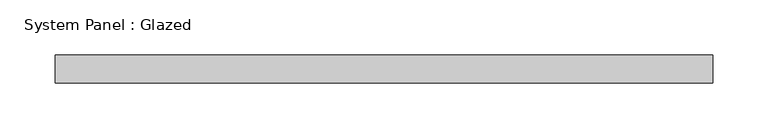
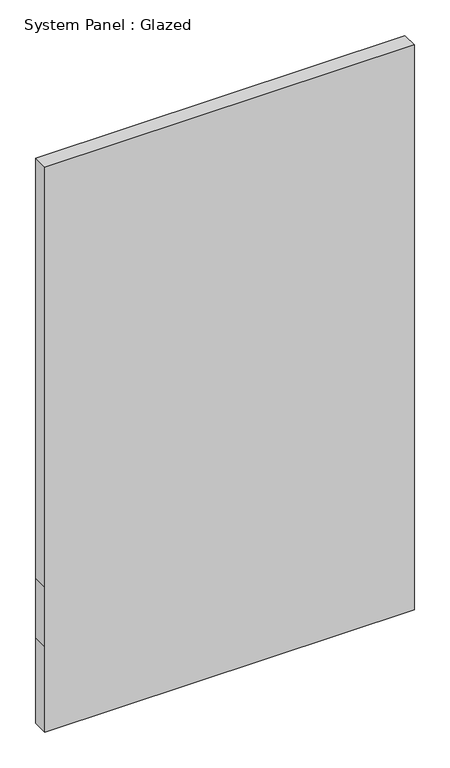
"""IFC4 building model written with IfcOpenShell, lengths in millimetres: plate geometry, System Panel : Glazed."""

from ifc_helpers import new_model, si_unit, frame, origin, place, context, project, spatial, polyline, outline, extrude, source, transform, mapped, element, save


def system_panel_glazed_6f1997f1(model_context):
    return source(origin(), model_context, "Body", "SweptSolid", [
        extrude(outline(polyline([(0.0, -298.45), (0.0, 298.45), (146.05, 298.45), (247.65, 298.45), (964.4309615, 298.45), (964.4309615, -298.45), (247.65, -298.45), (146.05, -298.45), (0.0, -298.45)])), frame((0.0, 19.05, 0.0), z_axis=(0.0, 1.0, 0.0), x_axis=(0.0, 0.0, 1.0)), (0.0, 0.0, 1.0), 25.4),
    ])


if __name__ == "__main__":
    model = new_model("IFC4")
    model_context = context("Model", 3, world=origin())
    ifc_project = project(units=[si_unit("LENGTHUNIT", "METRE", prefix="MILLI")], contexts=[model_context])
    site = spatial("IfcSite", under=ifc_project)
    building = spatial("IfcBuilding", under=site)
    placement = place(None, origin())
    system_panel_glazed_shape = system_panel_glazed_6f1997f1(model_context)
    element("IfcPlate", 1, ObjectType="System Panel : Glazed", at=placement, inside=building, context=model_context, shape_type="MappedRepresentation", body=[
        mapped(system_panel_glazed_shape, transform((0.0, 0.0, 0.0), x_axis=(1.0, 0.0, 0.0), y_axis=(0.0, 1.0, 0.0), z_axis=(0.0, 0.0, 1.0))),
    ])
    save(model, "model.ifc")

# Revit data of these elements
# Type "System Panel : Glazed"
#   Construction Type Id = "GSP4R"
#   Analytic Construction = "1/8 in Pilkington single glazing"
#   Visual Light Transmittance = 0.9
#   Solar Heat Gain Coefficient = 0.86
#   Heat Transfer Coefficient (U) = 1.18115 BTU/(h·ft²·°F)
#   Define Thermal Properties by = 1
# Element 1 (IfcPlate, "System Panel : Glazed")
#   Materials on its faces: "Glass"
# Materials
#   "Glass": class "Glass", colour RGB 0 128 192, transparency 0.75, Description = "Soda Lime Glass", Cost = 0
